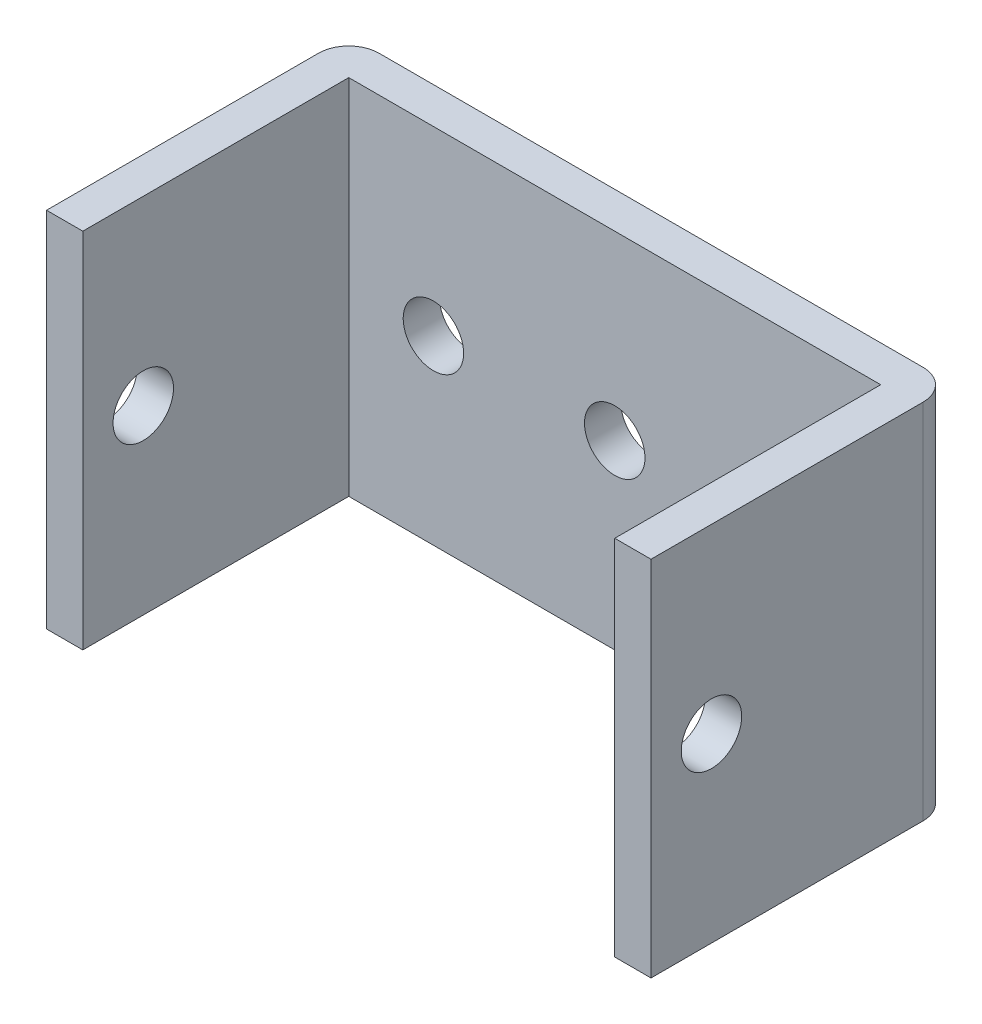
ISO-10303-21;
HEADER;
FILE_DESCRIPTION(('STEP AP214'),'2;1');
FILE_NAME('part.step','',(''),(''),'','','');
FILE_SCHEMA(('AUTOMOTIVE_DESIGN { 1 0 10303 214 1 1 1 1 }'));
ENDSEC;
DATA;
#1=APPLICATION_CONTEXT('core data for automotive mechanical design processes');
#2=APPLICATION_PROTOCOL_DEFINITION('international standard','automotive_design',2000,#1);
#3=PRODUCT_CONTEXT('',#1,'mechanical');
#4=PRODUCT('Part','Part','',(#3));
#5=PRODUCT_RELATED_PRODUCT_CATEGORY('part','',(#4));
#6=PRODUCT_DEFINITION_FORMATION('','',#4);
#7=PRODUCT_DEFINITION_CONTEXT('part definition',#1,'design');
#8=PRODUCT_DEFINITION('design','',#6,#7);
#9=PRODUCT_DEFINITION_SHAPE('','',#8);
#10=(LENGTH_UNIT() NAMED_UNIT(*) SI_UNIT(.MILLI.,.METRE.));
#11=(NAMED_UNIT(*) PLANE_ANGLE_UNIT() SI_UNIT($,.RADIAN.));
#12=(NAMED_UNIT(*) SI_UNIT($,.STERADIAN.) SOLID_ANGLE_UNIT());
#13=UNCERTAINTY_MEASURE_WITH_UNIT(LENGTH_MEASURE(1.E-05),#10,'distance_accuracy_value','');
#14=(GEOMETRIC_REPRESENTATION_CONTEXT(3) GLOBAL_UNCERTAINTY_ASSIGNED_CONTEXT((#13)) GLOBAL_UNIT_ASSIGNED_CONTEXT((#10,
#11,#12)) REPRESENTATION_CONTEXT('',''));
#15=CARTESIAN_POINT('',(0.,0.,0.));
#16=DIRECTION('',(0.,0.,1.));
#17=DIRECTION('',(1.,0.,0.));
#18=AXIS2_PLACEMENT_3D('',#15,#16,#17);
#19=CARTESIAN_POINT('',(6.,-30.,0.));
#20=DIRECTION('',(0.,0.,1.));
#21=DIRECTION('',(1.,0.,0.));
#22=AXIS2_PLACEMENT_3D('',#19,#20,#21);
#23=PLANE('',#22);
#24=DIRECTION('',(1.,0.,0.));
#25=VECTOR('',#24,1.);
#26=CARTESIAN_POINT('',(6.,30.,0.));
#27=LINE('',#26,#25);
#28=CARTESIAN_POINT('',(0.,30.,0.));
#29=VERTEX_POINT('',#28);
#30=CARTESIAN_POINT('',(6.,30.,0.));
#31=VERTEX_POINT('',#30);
#32=EDGE_CURVE('E161',#29,#31,#27,.T.);
#33=ORIENTED_EDGE('',*,*,#32,.F.);
#34=DIRECTION('',(0.,1.,0.));
#35=VECTOR('',#34,1.);
#36=CARTESIAN_POINT('',(0.,-30.,0.));
#37=LINE('',#36,#35);
#38=CARTESIAN_POINT('',(0.,-30.,0.));
#39=VERTEX_POINT('',#38);
#40=EDGE_CURVE('E138',#39,#29,#37,.T.);
#41=ORIENTED_EDGE('',*,*,#40,.F.);
#42=DIRECTION('',(1.,0.,0.));
#43=VECTOR('',#42,1.);
#44=CARTESIAN_POINT('',(6.,-30.,0.));
#45=LINE('',#44,#43);
#46=CARTESIAN_POINT('',(6.,-30.,0.));
#47=VERTEX_POINT('',#46);
#48=EDGE_CURVE('E132',#39,#47,#45,.T.);
#49=ORIENTED_EDGE('',*,*,#48,.T.);
#50=DIRECTION('',(0.,1.,0.));
#51=VECTOR('',#50,1.);
#52=CARTESIAN_POINT('',(6.,-30.,0.));
#53=LINE('',#52,#51);
#54=EDGE_CURVE('E116',#47,#31,#53,.T.);
#55=ORIENTED_EDGE('',*,*,#54,.T.);
#56=EDGE_LOOP('',(#33,#41,#49,#55));
#57=FACE_BOUND('',#56,.T.);
#58=ADVANCED_FACE('F39',(#57),#23,.T.);
#59=CARTESIAN_POINT('',(0.,-30.,0.));
#60=DIRECTION('',(-1.,0.,0.));
#61=DIRECTION('',(0.,0.,1.));
#62=AXIS2_PLACEMENT_3D('',#59,#60,#61);
#63=PLANE('',#62);
#64=CARTESIAN_POINT('',(0.,0.,-10.));
#65=DIRECTION('',(-1.,0.,0.));
#66=DIRECTION('',(0.,0.,1.));
#67=AXIS2_PLACEMENT_3D('',#64,#65,#66);
#68=CIRCLE('',#67,5.);
#69=CARTESIAN_POINT('',(0.,0.,-15.));
#70=VERTEX_POINT('',#69);
#71=EDGE_CURVE('E205',#70,#70,#68,.F.);
#72=ORIENTED_EDGE('',*,*,#71,.T.);
#73=EDGE_LOOP('',(#72));
#74=FACE_BOUND('',#73,.T.);
#75=DIRECTION('',(0.,0.,1.));
#76=VECTOR('',#75,1.);
#77=CARTESIAN_POINT('',(0.,30.,0.));
#78=LINE('',#77,#76);
#79=CARTESIAN_POINT('',(0.,30.,-45.));
#80=VERTEX_POINT('',#79);
#81=EDGE_CURVE('E139',#80,#29,#78,.T.);
#82=ORIENTED_EDGE('',*,*,#81,.F.);
#83=DIRECTION('',(0.,1.,0.));
#84=VECTOR('',#83,1.);
#85=CARTESIAN_POINT('',(0.,-30.,-45.));
#86=LINE('',#85,#84);
#87=CARTESIAN_POINT('',(0.,-30.,-45.));
#88=VERTEX_POINT('',#87);
#89=EDGE_CURVE('E11',#80,#88,#86,.F.);
#90=ORIENTED_EDGE('',*,*,#89,.T.);
#91=DIRECTION('',(0.,0.,1.));
#92=VECTOR('',#91,1.);
#93=CARTESIAN_POINT('',(0.,-30.,0.));
#94=LINE('',#93,#92);
#95=EDGE_CURVE('E130',#88,#39,#94,.T.);
#96=ORIENTED_EDGE('',*,*,#95,.T.);
#97=ORIENTED_EDGE('',*,*,#40,.T.);
#98=EDGE_LOOP('',(#82,#90,#96,#97));
#99=FACE_BOUND('',#98,.T.);
#100=ADVANCED_FACE('F231',(#74,#99),#63,.T.);
#101=CARTESIAN_POINT('',(0.,-30.,-50.));
#102=DIRECTION('',(0.,0.,-1.));
#103=DIRECTION('',(-1.,0.,0.));
#104=AXIS2_PLACEMENT_3D('',#101,#102,#103);
#105=PLANE('',#104);
#106=CARTESIAN_POINT('',(80.,0.,-50.));
#107=DIRECTION('',(0.,0.,-1.));
#108=DIRECTION('',(-1.,0.,0.));
#109=AXIS2_PLACEMENT_3D('',#106,#107,#108);
#110=CIRCLE('',#109,4.99999999999999);
#111=CARTESIAN_POINT('',(75.,0.,-50.));
#112=VERTEX_POINT('',#111);
#113=EDGE_CURVE('E144',#112,#112,#110,.T.);
#114=ORIENTED_EDGE('',*,*,#113,.F.);
#115=EDGE_LOOP('',(#114));
#116=FACE_BOUND('',#115,.T.);
#117=CARTESIAN_POINT('',(20.,0.,-50.));
#118=DIRECTION('',(0.,0.,-1.));
#119=DIRECTION('',(-1.,0.,0.));
#120=AXIS2_PLACEMENT_3D('',#117,#118,#119);
#121=CIRCLE('',#120,5.);
#122=CARTESIAN_POINT('',(15.,0.,-50.));
#123=VERTEX_POINT('',#122);
#124=EDGE_CURVE('E194',#123,#123,#121,.T.);
#125=ORIENTED_EDGE('',*,*,#124,.F.);
#126=EDGE_LOOP('',(#125));
#127=FACE_BOUND('',#126,.T.);
#128=CARTESIAN_POINT('',(50.,0.,-50.));
#129=DIRECTION('',(0.,0.,-1.));
#130=DIRECTION('',(-1.,0.,0.));
#131=AXIS2_PLACEMENT_3D('',#128,#129,#130);
#132=CIRCLE('',#131,5.00000000000002);
#133=CARTESIAN_POINT('',(45.,0.,-50.));
#134=VERTEX_POINT('',#133);
#135=EDGE_CURVE('E190',#134,#134,#132,.T.);
#136=ORIENTED_EDGE('',*,*,#135,.F.);
#137=EDGE_LOOP('',(#136));
#138=FACE_BOUND('',#137,.T.);
#139=DIRECTION('',(-1.,0.,0.));
#140=VECTOR('',#139,1.);
#141=CARTESIAN_POINT('',(0.,30.,-50.));
#142=LINE('',#141,#140);
#143=CARTESIAN_POINT('',(95.,30.,-50.));
#144=VERTEX_POINT('',#143);
#145=CARTESIAN_POINT('',(5.,30.,-50.));
#146=VERTEX_POINT('',#145);
#147=EDGE_CURVE('E142',#144,#146,#142,.T.);
#148=ORIENTED_EDGE('',*,*,#147,.F.);
#149=DIRECTION('',(0.,1.,0.));
#150=VECTOR('',#149,1.);
#151=CARTESIAN_POINT('',(95.,-30.,-50.));
#152=LINE('',#151,#150);
#153=CARTESIAN_POINT('',(95.,-30.,-50.));
#154=VERTEX_POINT('',#153);
#155=EDGE_CURVE('E215',#144,#154,#152,.F.);
#156=ORIENTED_EDGE('',*,*,#155,.T.);
#157=DIRECTION('',(-1.,0.,0.));
#158=VECTOR('',#157,1.);
#159=CARTESIAN_POINT('',(0.,-30.,-50.));
#160=LINE('',#159,#158);
#161=CARTESIAN_POINT('',(5.,-30.,-50.));
#162=VERTEX_POINT('',#161);
#163=EDGE_CURVE('E158',#154,#162,#160,.T.);
#164=ORIENTED_EDGE('',*,*,#163,.T.);
#165=DIRECTION('',(0.,1.,0.));
#166=VECTOR('',#165,1.);
#167=CARTESIAN_POINT('',(5.,-30.,-50.));
#168=LINE('',#167,#166);
#169=EDGE_CURVE('E207',#162,#146,#168,.T.);
#170=ORIENTED_EDGE('',*,*,#169,.T.);
#171=EDGE_LOOP('',(#148,#156,#164,#170));
#172=FACE_BOUND('',#171,.T.);
#173=ADVANCED_FACE('F229',(#116,#127,#138,#172),#105,.T.);
#174=CARTESIAN_POINT('',(100.,-30.,-50.));
#175=DIRECTION('',(1.,0.,0.));
#176=DIRECTION('',(0.,0.,-1.));
#177=AXIS2_PLACEMENT_3D('',#174,#175,#176);
#178=PLANE('',#177);
#179=CARTESIAN_POINT('',(100.,0.,-10.));
#180=DIRECTION('',(1.,0.,0.));
#181=DIRECTION('',(0.,0.,-1.));
#182=AXIS2_PLACEMENT_3D('',#179,#180,#181);
#183=CIRCLE('',#182,5.);
#184=CARTESIAN_POINT('',(100.,0.,-15.));
#185=VERTEX_POINT('',#184);
#186=EDGE_CURVE('E330',#185,#185,#183,.T.);
#187=ORIENTED_EDGE('',*,*,#186,.F.);
#188=EDGE_LOOP('',(#187));
#189=FACE_BOUND('',#188,.T.);
#190=DIRECTION('',(0.,0.,-1.));
#191=VECTOR('',#190,1.);
#192=CARTESIAN_POINT('',(100.,-30.,-50.));
#193=LINE('',#192,#191);
#194=CARTESIAN_POINT('',(100.,-30.,0.));
#195=VERTEX_POINT('',#194);
#196=CARTESIAN_POINT('',(100.,-30.,-45.));
#197=VERTEX_POINT('',#196);
#198=EDGE_CURVE('E154',#195,#197,#193,.T.);
#199=ORIENTED_EDGE('',*,*,#198,.T.);
#200=DIRECTION('',(0.,1.,0.));
#201=VECTOR('',#200,1.);
#202=CARTESIAN_POINT('',(100.,-30.,-45.));
#203=LINE('',#202,#201);
#204=CARTESIAN_POINT('',(100.,30.,-45.));
#205=VERTEX_POINT('',#204);
#206=EDGE_CURVE('E178',#197,#205,#203,.T.);
#207=ORIENTED_EDGE('',*,*,#206,.T.);
#208=DIRECTION('',(0.,0.,-1.));
#209=VECTOR('',#208,1.);
#210=CARTESIAN_POINT('',(100.,30.,-50.));
#211=LINE('',#210,#209);
#212=CARTESIAN_POINT('',(100.,30.,0.));
#213=VERTEX_POINT('',#212);
#214=EDGE_CURVE('E174',#213,#205,#211,.T.);
#215=ORIENTED_EDGE('',*,*,#214,.F.);
#216=DIRECTION('',(0.,1.,0.));
#217=VECTOR('',#216,1.);
#218=CARTESIAN_POINT('',(100.,-30.,0.));
#219=LINE('',#218,#217);
#220=EDGE_CURVE('E179',#195,#213,#219,.T.);
#221=ORIENTED_EDGE('',*,*,#220,.F.);
#222=EDGE_LOOP('',(#199,#207,#215,#221));
#223=FACE_BOUND('',#222,.T.);
#224=ADVANCED_FACE('F222',(#189,#223),#178,.T.);
#225=CARTESIAN_POINT('',(100.,-30.,0.));
#226=DIRECTION('',(0.,0.,1.));
#227=DIRECTION('',(1.,0.,0.));
#228=AXIS2_PLACEMENT_3D('',#225,#226,#227);
#229=PLANE('',#228);
#230=DIRECTION('',(1.,0.,0.));
#231=VECTOR('',#230,1.);
#232=CARTESIAN_POINT('',(100.,30.,0.));
#233=LINE('',#232,#231);
#234=CARTESIAN_POINT('',(94.,30.,0.));
#235=VERTEX_POINT('',#234);
#236=EDGE_CURVE('E168',#235,#213,#233,.T.);
#237=ORIENTED_EDGE('',*,*,#236,.F.);
#238=DIRECTION('',(0.,1.,0.));
#239=VECTOR('',#238,1.);
#240=CARTESIAN_POINT('',(94.,-30.,0.));
#241=LINE('',#240,#239);
#242=CARTESIAN_POINT('',(94.,-30.,0.));
#243=VERTEX_POINT('',#242);
#244=EDGE_CURVE('E185',#243,#235,#241,.T.);
#245=ORIENTED_EDGE('',*,*,#244,.F.);
#246=DIRECTION('',(1.,0.,0.));
#247=VECTOR('',#246,1.);
#248=CARTESIAN_POINT('',(100.,-30.,0.));
#249=LINE('',#248,#247);
#250=EDGE_CURVE('E155',#243,#195,#249,.T.);
#251=ORIENTED_EDGE('',*,*,#250,.T.);
#252=ORIENTED_EDGE('',*,*,#220,.T.);
#253=EDGE_LOOP('',(#237,#245,#251,#252));
#254=FACE_BOUND('',#253,.T.);
#255=ADVANCED_FACE('F238',(#254),#229,.T.);
#256=CARTESIAN_POINT('',(94.,-30.,0.));
#257=DIRECTION('',(-1.,0.,0.));
#258=DIRECTION('',(0.,0.,1.));
#259=AXIS2_PLACEMENT_3D('',#256,#257,#258);
#260=PLANE('',#259);
#261=CARTESIAN_POINT('',(94.,0.,-10.));
#262=DIRECTION('',(-1.,0.,0.));
#263=DIRECTION('',(0.,0.,1.));
#264=AXIS2_PLACEMENT_3D('',#261,#262,#263);
#265=CIRCLE('',#264,5.);
#266=CARTESIAN_POINT('',(94.,0.,-15.));
#267=VERTEX_POINT('',#266);
#268=EDGE_CURVE('E191',#267,#267,#265,.T.);
#269=ORIENTED_EDGE('',*,*,#268,.F.);
#270=EDGE_LOOP('',(#269));
#271=FACE_BOUND('',#270,.T.);
#272=DIRECTION('',(0.,0.,1.));
#273=VECTOR('',#272,1.);
#274=CARTESIAN_POINT('',(94.,30.,0.));
#275=LINE('',#274,#273);
#276=CARTESIAN_POINT('',(94.,30.,-44.));
#277=VERTEX_POINT('',#276);
#278=EDGE_CURVE('E170',#277,#235,#275,.T.);
#279=ORIENTED_EDGE('',*,*,#278,.F.);
#280=DIRECTION('',(0.,1.,0.));
#281=VECTOR('',#280,1.);
#282=CARTESIAN_POINT('',(94.,-30.,-44.));
#283=LINE('',#282,#281);
#284=CARTESIAN_POINT('',(94.,-30.,-44.));
#285=VERTEX_POINT('',#284);
#286=EDGE_CURVE('E184',#285,#277,#283,.T.);
#287=ORIENTED_EDGE('',*,*,#286,.F.);
#288=DIRECTION('',(0.,0.,1.));
#289=VECTOR('',#288,1.);
#290=CARTESIAN_POINT('',(94.,-30.,0.));
#291=LINE('',#290,#289);
#292=EDGE_CURVE('E149',#285,#243,#291,.T.);
#293=ORIENTED_EDGE('',*,*,#292,.T.);
#294=ORIENTED_EDGE('',*,*,#244,.T.);
#295=EDGE_LOOP('',(#279,#287,#293,#294));
#296=FACE_BOUND('',#295,.T.);
#297=ADVANCED_FACE('F240',(#271,#296),#260,.T.);
#298=CARTESIAN_POINT('',(94.,-30.,-44.));
#299=DIRECTION('',(0.,0.,1.));
#300=DIRECTION('',(1.,0.,0.));
#301=AXIS2_PLACEMENT_3D('',#298,#299,#300);
#302=PLANE('',#301);
#303=CARTESIAN_POINT('',(80.,0.,-44.));
#304=DIRECTION('',(0.,0.,1.));
#305=DIRECTION('',(1.,0.,0.));
#306=AXIS2_PLACEMENT_3D('',#303,#304,#305);
#307=CIRCLE('',#306,4.99999999999999);
#308=CARTESIAN_POINT('',(85.,0.,-44.));
#309=VERTEX_POINT('',#308);
#310=EDGE_CURVE('E198',#309,#309,#307,.T.);
#311=ORIENTED_EDGE('',*,*,#310,.F.);
#312=EDGE_LOOP('',(#311));
#313=FACE_BOUND('',#312,.T.);
#314=CARTESIAN_POINT('',(20.,0.,-44.));
#315=DIRECTION('',(0.,0.,1.));
#316=DIRECTION('',(1.,0.,0.));
#317=AXIS2_PLACEMENT_3D('',#314,#315,#316);
#318=CIRCLE('',#317,5.);
#319=CARTESIAN_POINT('',(25.,0.,-44.));
#320=VERTEX_POINT('',#319);
#321=EDGE_CURVE('E195',#320,#320,#318,.T.);
#322=ORIENTED_EDGE('',*,*,#321,.F.);
#323=EDGE_LOOP('',(#322));
#324=FACE_BOUND('',#323,.T.);
#325=CARTESIAN_POINT('',(50.,0.,-44.));
#326=DIRECTION('',(0.,0.,1.));
#327=DIRECTION('',(1.,0.,0.));
#328=AXIS2_PLACEMENT_3D('',#325,#326,#327);
#329=CIRCLE('',#328,5.00000000000002);
#330=CARTESIAN_POINT('',(55.,0.,-44.));
#331=VERTEX_POINT('',#330);
#332=EDGE_CURVE('E187',#331,#331,#329,.T.);
#333=ORIENTED_EDGE('',*,*,#332,.F.);
#334=EDGE_LOOP('',(#333));
#335=FACE_BOUND('',#334,.T.);
#336=DIRECTION('',(1.,0.,0.));
#337=VECTOR('',#336,1.);
#338=CARTESIAN_POINT('',(94.,30.,-44.));
#339=LINE('',#338,#337);
#340=CARTESIAN_POINT('',(6.00000000000001,30.,-44.));
#341=VERTEX_POINT('',#340);
#342=EDGE_CURVE('E163',#341,#277,#339,.T.);
#343=ORIENTED_EDGE('',*,*,#342,.F.);
#344=DIRECTION('',(0.,1.,0.));
#345=VECTOR('',#344,1.);
#346=CARTESIAN_POINT('',(6.00000000000001,-30.,-44.));
#347=LINE('',#346,#345);
#348=CARTESIAN_POINT('',(6.00000000000001,-30.,-44.));
#349=VERTEX_POINT('',#348);
#350=EDGE_CURVE('E127',#349,#341,#347,.T.);
#351=ORIENTED_EDGE('',*,*,#350,.F.);
#352=DIRECTION('',(1.,0.,0.));
#353=VECTOR('',#352,1.);
#354=CARTESIAN_POINT('',(94.,-30.,-44.));
#355=LINE('',#354,#353);
#356=EDGE_CURVE('E135',#349,#285,#355,.T.);
#357=ORIENTED_EDGE('',*,*,#356,.T.);
#358=ORIENTED_EDGE('',*,*,#286,.T.);
#359=EDGE_LOOP('',(#343,#351,#357,#358));
#360=FACE_BOUND('',#359,.T.);
#361=ADVANCED_FACE('F234',(#313,#324,#335,#360),#302,.T.);
#362=CARTESIAN_POINT('',(6.00000000000001,-30.,-44.));
#363=DIRECTION('',(1.,0.,0.));
#364=DIRECTION('',(0.,0.,-1.));
#365=AXIS2_PLACEMENT_3D('',#362,#363,#364);
#366=PLANE('',#365);
#367=CARTESIAN_POINT('',(6.00000000000001,0.,-10.));
#368=DIRECTION('',(1.,0.,0.));
#369=DIRECTION('',(0.,0.,-1.));
#370=AXIS2_PLACEMENT_3D('',#367,#368,#369);
#371=CIRCLE('',#370,5.);
#372=CARTESIAN_POINT('',(6.00000000000001,0.,-15.));
#373=VERTEX_POINT('',#372);
#374=EDGE_CURVE('E200',#373,#373,#371,.T.);
#375=ORIENTED_EDGE('',*,*,#374,.F.);
#376=EDGE_LOOP('',(#375));
#377=FACE_BOUND('',#376,.T.);
#378=DIRECTION('',(0.,0.,-1.));
#379=VECTOR('',#378,1.);
#380=CARTESIAN_POINT('',(6.00000000000001,30.,-44.));
#381=LINE('',#380,#379);
#382=EDGE_CURVE('E121',#31,#341,#381,.T.);
#383=ORIENTED_EDGE('',*,*,#382,.F.);
#384=ORIENTED_EDGE('',*,*,#54,.F.);
#385=DIRECTION('',(0.,0.,-1.));
#386=VECTOR('',#385,1.);
#387=CARTESIAN_POINT('',(6.00000000000001,-30.,-44.));
#388=LINE('',#387,#386);
#389=EDGE_CURVE('E118',#47,#349,#388,.T.);
#390=ORIENTED_EDGE('',*,*,#389,.T.);
#391=ORIENTED_EDGE('',*,*,#350,.T.);
#392=EDGE_LOOP('',(#383,#384,#390,#391));
#393=FACE_BOUND('',#392,.T.);
#394=ADVANCED_FACE('F119',(#377,#393),#366,.T.);
#395=CARTESIAN_POINT('',(0.,-30.,0.));
#396=DIRECTION('',(0.,-1.,0.));
#397=DIRECTION('',(0.,0.,-1.));
#398=AXIS2_PLACEMENT_3D('',#395,#396,#397);
#399=PLANE('',#398);
#400=ORIENTED_EDGE('',*,*,#163,.F.);
#401=CARTESIAN_POINT('',(95.,-30.,-45.));
#402=DIRECTION('',(0.,-1.,0.));
#403=DIRECTION('',(0.,0.,-1.));
#404=AXIS2_PLACEMENT_3D('',#401,#402,#403);
#405=CIRCLE('',#404,5.);
#406=EDGE_CURVE('E50',#154,#197,#405,.T.);
#407=ORIENTED_EDGE('',*,*,#406,.T.);
#408=ORIENTED_EDGE('',*,*,#198,.F.);
#409=ORIENTED_EDGE('',*,*,#250,.F.);
#410=ORIENTED_EDGE('',*,*,#292,.F.);
#411=ORIENTED_EDGE('',*,*,#356,.F.);
#412=ORIENTED_EDGE('',*,*,#389,.F.);
#413=ORIENTED_EDGE('',*,*,#48,.F.);
#414=ORIENTED_EDGE('',*,*,#95,.F.);
#415=CARTESIAN_POINT('',(5.,-30.,-45.));
#416=DIRECTION('',(0.,-1.,0.));
#417=DIRECTION('',(0.,0.,-1.));
#418=AXIS2_PLACEMENT_3D('',#415,#416,#417);
#419=CIRCLE('',#418,5.);
#420=EDGE_CURVE('E56',#88,#162,#419,.T.);
#421=ORIENTED_EDGE('',*,*,#420,.T.);
#422=EDGE_LOOP('',(#400,#407,#408,#409,#410,#411,#412,#413,#414,#421));
#423=FACE_BOUND('',#422,.T.);
#424=ADVANCED_FACE('F131',(#423),#399,.T.);
#425=CARTESIAN_POINT('',(0.,30.,0.));
#426=DIRECTION('',(0.,-1.,0.));
#427=DIRECTION('',(0.,0.,-1.));
#428=AXIS2_PLACEMENT_3D('',#425,#426,#427);
#429=PLANE('',#428);
#430=ORIENTED_EDGE('',*,*,#214,.T.);
#431=CARTESIAN_POINT('',(95.,30.,-45.));
#432=DIRECTION('',(0.,-1.,0.));
#433=DIRECTION('',(0.,0.,-1.));
#434=AXIS2_PLACEMENT_3D('',#431,#432,#433);
#435=CIRCLE('',#434,5.);
#436=EDGE_CURVE('E210',#205,#144,#435,.F.);
#437=ORIENTED_EDGE('',*,*,#436,.T.);
#438=ORIENTED_EDGE('',*,*,#147,.T.);
#439=CARTESIAN_POINT('',(5.,30.,-45.));
#440=DIRECTION('',(0.,-1.,0.));
#441=DIRECTION('',(0.,0.,-1.));
#442=AXIS2_PLACEMENT_3D('',#439,#440,#441);
#443=CIRCLE('',#442,5.);
#444=EDGE_CURVE('E202',#146,#80,#443,.F.);
#445=ORIENTED_EDGE('',*,*,#444,.T.);
#446=ORIENTED_EDGE('',*,*,#81,.T.);
#447=ORIENTED_EDGE('',*,*,#32,.T.);
#448=ORIENTED_EDGE('',*,*,#382,.T.);
#449=ORIENTED_EDGE('',*,*,#342,.T.);
#450=ORIENTED_EDGE('',*,*,#278,.T.);
#451=ORIENTED_EDGE('',*,*,#236,.T.);
#452=EDGE_LOOP('',(#430,#437,#438,#445,#446,#447,#448,#449,#450,#451));
#453=FACE_BOUND('',#452,.T.);
#454=ADVANCED_FACE('F226',(#453),#429,.F.);
#455=CARTESIAN_POINT('',(50.,0.,-20.));
#456=DIRECTION('',(0.,0.,-1.));
#457=DIRECTION('',(-1.,0.,0.));
#458=AXIS2_PLACEMENT_3D('',#455,#456,#457);
#459=CYLINDRICAL_SURFACE('',#458,5.00000000000002);
#460=ORIENTED_EDGE('',*,*,#135,.T.);
#461=EDGE_LOOP('',(#460));
#462=FACE_BOUND('',#461,.T.);
#463=ORIENTED_EDGE('',*,*,#332,.T.);
#464=EDGE_LOOP('',(#463));
#465=FACE_BOUND('',#464,.T.);
#466=ADVANCED_FACE('F282',(#462,#465),#459,.F.);
#467=CARTESIAN_POINT('',(20.,0.,-20.));
#468=DIRECTION('',(0.,0.,-1.));
#469=DIRECTION('',(-1.,0.,0.));
#470=AXIS2_PLACEMENT_3D('',#467,#468,#469);
#471=CYLINDRICAL_SURFACE('',#470,5.);
#472=ORIENTED_EDGE('',*,*,#124,.T.);
#473=EDGE_LOOP('',(#472));
#474=FACE_BOUND('',#473,.T.);
#475=ORIENTED_EDGE('',*,*,#321,.T.);
#476=EDGE_LOOP('',(#475));
#477=FACE_BOUND('',#476,.T.);
#478=ADVANCED_FACE('F276',(#474,#477),#471,.F.);
#479=CARTESIAN_POINT('',(80.,0.,-20.));
#480=DIRECTION('',(0.,0.,-1.));
#481=DIRECTION('',(-1.,0.,0.));
#482=AXIS2_PLACEMENT_3D('',#479,#480,#481);
#483=CYLINDRICAL_SURFACE('',#482,4.99999999999999);
#484=ORIENTED_EDGE('',*,*,#113,.T.);
#485=EDGE_LOOP('',(#484));
#486=FACE_BOUND('',#485,.T.);
#487=ORIENTED_EDGE('',*,*,#310,.T.);
#488=EDGE_LOOP('',(#487));
#489=FACE_BOUND('',#488,.T.);
#490=ADVANCED_FACE('F273',(#486,#489),#483,.F.);
#491=CARTESIAN_POINT('',(-14.142135623731,0.,-10.));
#492=DIRECTION('',(1.,0.,0.));
#493=DIRECTION('',(0.,0.,-1.));
#494=AXIS2_PLACEMENT_3D('',#491,#492,#493);
#495=CYLINDRICAL_SURFACE('',#494,5.);
#496=CARTESIAN_POINT('',(6.00000000000001,0.,-15.));
#497=CARTESIAN_POINT('',(5.93750000000001,0.,-15.));
#498=CARTESIAN_POINT('',(5.87500000000001,0.,-15.));
#499=CARTESIAN_POINT('',(5.75000000000001,0.,-15.));
#500=CARTESIAN_POINT('',(5.68750000000001,0.,-15.));
#501=CARTESIAN_POINT('',(5.56250000000001,0.,-15.));
#502=CARTESIAN_POINT('',(5.50000000000001,0.,-15.));
#503=CARTESIAN_POINT('',(5.37500000000001,0.,-15.));
#504=CARTESIAN_POINT('',(5.31250000000001,0.,-15.));
#505=CARTESIAN_POINT('',(5.18750000000001,0.,-15.));
#506=CARTESIAN_POINT('',(5.12500000000001,0.,-15.));
#507=CARTESIAN_POINT('',(5.00000000000001,0.,-15.));
#508=CARTESIAN_POINT('',(4.93750000000001,0.,-15.));
#509=CARTESIAN_POINT('',(4.81250000000001,0.,-15.));
#510=CARTESIAN_POINT('',(4.75000000000001,0.,-15.));
#511=CARTESIAN_POINT('',(4.62500000000001,0.,-15.));
#512=CARTESIAN_POINT('',(4.56250000000001,0.,-15.));
#513=CARTESIAN_POINT('',(4.43750000000001,0.,-15.));
#514=CARTESIAN_POINT('',(4.37500000000001,0.,-15.));
#515=CARTESIAN_POINT('',(4.25000000000001,0.,-15.));
#516=CARTESIAN_POINT('',(4.18750000000001,0.,-15.));
#517=CARTESIAN_POINT('',(4.06250000000001,0.,-15.));
#518=CARTESIAN_POINT('',(4.00000000000001,0.,-15.));
#519=CARTESIAN_POINT('',(3.87500000000001,0.,-15.));
#520=CARTESIAN_POINT('',(3.81250000000001,0.,-15.));
#521=CARTESIAN_POINT('',(3.68750000000001,0.,-15.));
#522=CARTESIAN_POINT('',(3.62500000000001,0.,-15.));
#523=CARTESIAN_POINT('',(3.50000000000001,0.,-15.));
#524=CARTESIAN_POINT('',(3.43750000000001,0.,-15.));
#525=CARTESIAN_POINT('',(3.31250000000001,0.,-15.));
#526=CARTESIAN_POINT('',(3.25000000000001,0.,-15.));
#527=CARTESIAN_POINT('',(3.12500000000001,0.,-15.));
#528=CARTESIAN_POINT('',(3.06250000000001,0.,-15.));
#529=CARTESIAN_POINT('',(2.93750000000001,0.,-15.));
#530=CARTESIAN_POINT('',(2.87500000000001,0.,-15.));
#531=CARTESIAN_POINT('',(2.75000000000001,0.,-15.));
#532=CARTESIAN_POINT('',(2.68750000000001,0.,-15.));
#533=CARTESIAN_POINT('',(2.5625,0.,-15.));
#534=CARTESIAN_POINT('',(2.5,0.,-15.));
#535=CARTESIAN_POINT('',(2.375,0.,-15.));
#536=CARTESIAN_POINT('',(2.3125,0.,-15.));
#537=CARTESIAN_POINT('',(2.1875,0.,-15.));
#538=CARTESIAN_POINT('',(2.125,0.,-15.));
#539=CARTESIAN_POINT('',(2.,0.,-15.));
#540=CARTESIAN_POINT('',(1.9375,0.,-15.));
#541=CARTESIAN_POINT('',(1.8125,0.,-15.));
#542=CARTESIAN_POINT('',(1.75,0.,-15.));
#543=CARTESIAN_POINT('',(1.625,0.,-15.));
#544=CARTESIAN_POINT('',(1.5625,0.,-15.));
#545=CARTESIAN_POINT('',(1.4375,0.,-15.));
#546=CARTESIAN_POINT('',(1.375,0.,-15.));
#547=CARTESIAN_POINT('',(1.25,0.,-15.));
#548=CARTESIAN_POINT('',(1.1875,0.,-15.));
#549=CARTESIAN_POINT('',(1.0625,0.,-15.));
#550=CARTESIAN_POINT('',(1.,0.,-15.));
#551=CARTESIAN_POINT('',(0.875000000000003,0.,-15.));
#552=CARTESIAN_POINT('',(0.812500000000002,0.,-15.));
#553=CARTESIAN_POINT('',(0.687500000000002,0.,-15.));
#554=CARTESIAN_POINT('',(0.625000000000002,0.,-15.));
#555=CARTESIAN_POINT('',(0.500000000000002,0.,-15.));
#556=CARTESIAN_POINT('',(0.437500000000002,0.,-15.));
#557=CARTESIAN_POINT('',(0.312500000000002,0.,-15.));
#558=CARTESIAN_POINT('',(0.250000000000002,0.,-15.));
#559=CARTESIAN_POINT('',(0.125000000000002,0.,-15.));
#560=CARTESIAN_POINT('',(0.0625000000000018,0.,-15.));
#561=CARTESIAN_POINT('',(0.,0.,-15.));
#562=B_SPLINE_CURVE_WITH_KNOTS('',3,(#496,#497,#498,#499,#500,#501,#502,#503,#504,#505,#506,
#507,#508,#509,#510,#511,#512,#513,#514,#515,#516,#517,#518,#519,#520,#521,#522,#523,#524,#525,
#526,#527,#528,#529,#530,#531,#532,#533,#534,#535,#536,#537,#538,#539,#540,#541,#542,#543,#544,
#545,#546,#547,#548,#549,#550,#551,#552,#553,#554,#555,#556,#557,#558,#559,#560,#561),
.UNSPECIFIED.,.F.,.F.,(4,2,2,2,2,2,2,2,2,2,2,2,2,2,2,2,2,2,2,2,2,2,2,2,2,2,2,2,2,2,2,2,4),(0.,
0.1875,0.375,0.5625,0.750000000000001,0.937500000000001,1.125,1.3125,1.5,1.6875,1.875,2.0625,
2.25,2.4375,2.625,2.8125,3.,3.1875,3.375,3.56250000000001,3.75000000000001,3.93750000000001,
4.12500000000001,4.31250000000001,4.50000000000001,4.68750000000001,4.87500000000001,
5.06250000000001,5.25000000000001,5.43750000000001,5.62500000000001,5.81250000000001,
6.00000000000001),.UNSPECIFIED.);
#563=EDGE_CURVE('BSEAM268',#373,#70,#562,.T.);
#564=ORIENTED_EDGE('',*,*,#374,.T.);
#565=ORIENTED_EDGE('',*,*,#71,.F.);
#566=ORIENTED_EDGE('',*,*,#563,.T.);
#567=ORIENTED_EDGE('',*,*,#563,.F.);
#568=EDGE_LOOP('',(#564,#566,#565,#567));
#569=FACE_BOUND('',#568,.T.);
#570=ADVANCED_FACE('F268',(#569),#495,.F.);
#571=CARTESIAN_POINT('',(94.,0.,-15.));
#572=CARTESIAN_POINT('',(94.0625,0.,-15.));
#573=CARTESIAN_POINT('',(94.125,0.,-15.));
#574=CARTESIAN_POINT('',(94.25,0.,-15.));
#575=CARTESIAN_POINT('',(94.3125,0.,-15.));
#576=CARTESIAN_POINT('',(94.4375,0.,-15.));
#577=CARTESIAN_POINT('',(94.5,0.,-15.));
#578=CARTESIAN_POINT('',(94.625,0.,-15.));
#579=CARTESIAN_POINT('',(94.6875,0.,-15.));
#580=CARTESIAN_POINT('',(94.8125,0.,-15.));
#581=CARTESIAN_POINT('',(94.875,0.,-15.));
#582=CARTESIAN_POINT('',(95.,0.,-15.));
#583=CARTESIAN_POINT('',(95.0625,0.,-15.));
#584=CARTESIAN_POINT('',(95.1875,0.,-15.));
#585=CARTESIAN_POINT('',(95.25,0.,-15.));
#586=CARTESIAN_POINT('',(95.375,0.,-15.));
#587=CARTESIAN_POINT('',(95.4375,0.,-15.));
#588=CARTESIAN_POINT('',(95.5625,0.,-15.));
#589=CARTESIAN_POINT('',(95.625,0.,-15.));
#590=CARTESIAN_POINT('',(95.75,0.,-15.));
#591=CARTESIAN_POINT('',(95.8125,0.,-15.));
#592=CARTESIAN_POINT('',(95.9375,0.,-15.));
#593=CARTESIAN_POINT('',(96.,0.,-15.));
#594=CARTESIAN_POINT('',(96.125,0.,-15.));
#595=CARTESIAN_POINT('',(96.1875,0.,-15.));
#596=CARTESIAN_POINT('',(96.3125,0.,-15.));
#597=CARTESIAN_POINT('',(96.375,0.,-15.));
#598=CARTESIAN_POINT('',(96.5,0.,-15.));
#599=CARTESIAN_POINT('',(96.5625,0.,-15.));
#600=CARTESIAN_POINT('',(96.6875,0.,-15.));
#601=CARTESIAN_POINT('',(96.75,0.,-15.));
#602=CARTESIAN_POINT('',(96.875,0.,-15.));
#603=CARTESIAN_POINT('',(96.9375,0.,-15.));
#604=CARTESIAN_POINT('',(97.0625,0.,-15.));
#605=CARTESIAN_POINT('',(97.125,0.,-15.));
#606=CARTESIAN_POINT('',(97.25,0.,-15.));
#607=CARTESIAN_POINT('',(97.3125,0.,-15.));
#608=CARTESIAN_POINT('',(97.4375,0.,-15.));
#609=CARTESIAN_POINT('',(97.5,0.,-15.));
#610=CARTESIAN_POINT('',(97.625,0.,-15.));
#611=CARTESIAN_POINT('',(97.6875,0.,-15.));
#612=CARTESIAN_POINT('',(97.8125,0.,-15.));
#613=CARTESIAN_POINT('',(97.875,0.,-15.));
#614=CARTESIAN_POINT('',(98.,0.,-15.));
#615=CARTESIAN_POINT('',(98.0625,0.,-15.));
#616=CARTESIAN_POINT('',(98.1875,0.,-15.));
#617=CARTESIAN_POINT('',(98.25,0.,-15.));
#618=CARTESIAN_POINT('',(98.375,0.,-15.));
#619=CARTESIAN_POINT('',(98.4375,0.,-15.));
#620=CARTESIAN_POINT('',(98.5625,0.,-15.));
#621=CARTESIAN_POINT('',(98.625,0.,-15.));
#622=CARTESIAN_POINT('',(98.75,0.,-15.));
#623=CARTESIAN_POINT('',(98.8125,0.,-15.));
#624=CARTESIAN_POINT('',(98.9375,0.,-15.));
#625=CARTESIAN_POINT('',(99.,0.,-15.));
#626=CARTESIAN_POINT('',(99.125,0.,-15.));
#627=CARTESIAN_POINT('',(99.1875,0.,-15.));
#628=CARTESIAN_POINT('',(99.3125,0.,-15.));
#629=CARTESIAN_POINT('',(99.375,0.,-15.));
#630=CARTESIAN_POINT('',(99.5,0.,-15.));
#631=CARTESIAN_POINT('',(99.5625,0.,-15.));
#632=CARTESIAN_POINT('',(99.6875,0.,-15.));
#633=CARTESIAN_POINT('',(99.75,0.,-15.));
#634=CARTESIAN_POINT('',(99.875,0.,-15.));
#635=CARTESIAN_POINT('',(99.9375,0.,-15.));
#636=CARTESIAN_POINT('',(100.,0.,-15.));
#637=B_SPLINE_CURVE_WITH_KNOTS('',3,(#571,#572,#573,#574,#575,#576,#577,#578,#579,#580,#581,
#582,#583,#584,#585,#586,#587,#588,#589,#590,#591,#592,#593,#594,#595,#596,#597,#598,#599,#600,
#601,#602,#603,#604,#605,#606,#607,#608,#609,#610,#611,#612,#613,#614,#615,#616,#617,#618,#619,
#620,#621,#622,#623,#624,#625,#626,#627,#628,#629,#630,#631,#632,#633,#634,#635,#636),
.UNSPECIFIED.,.F.,.F.,(4,2,2,2,2,2,2,2,2,2,2,2,2,2,2,2,2,2,2,2,2,2,2,2,2,2,2,2,2,2,2,2,4),(0.,
0.187499999999993,0.375,0.562499999999994,0.750000000000001,0.937499999999994,1.125,
1.31249999999999,1.5,1.68749999999999,1.87499999999999,2.06249999999999,2.24999999999999,2.4375,
2.62499999999999,2.8125,2.99999999999999,3.18749999999998,3.37499999999999,3.56249999999998,
3.74999999999999,3.93749999999998,4.12499999999999,4.31249999999998,4.49999999999998,
4.68749999999998,4.87499999999998,5.06249999999998,5.24999999999998,5.43749999999998,
5.62499999999998,5.81249999999998,5.99999999999998),.UNSPECIFIED.);
#638=EDGE_CURVE('BSEAM265',#267,#185,#637,.T.);
#639=ORIENTED_EDGE('',*,*,#268,.T.);
#640=ORIENTED_EDGE('',*,*,#186,.T.);
#641=ORIENTED_EDGE('',*,*,#638,.T.);
#642=ORIENTED_EDGE('',*,*,#638,.F.);
#643=EDGE_LOOP('',(#639,#641,#640,#642));
#644=FACE_BOUND('',#643,.T.);
#645=ADVANCED_FACE('F265',(#644),#495,.F.);
#646=CARTESIAN_POINT('',(95.,-30.,-45.));
#647=DIRECTION('',(0.,1.,0.));
#648=DIRECTION('',(0.,0.,1.));
#649=AXIS2_PLACEMENT_3D('',#646,#647,#648);
#650=CYLINDRICAL_SURFACE('',#649,5.);
#651=ORIENTED_EDGE('',*,*,#406,.F.);
#652=ORIENTED_EDGE('',*,*,#155,.F.);
#653=ORIENTED_EDGE('',*,*,#436,.F.);
#654=ORIENTED_EDGE('',*,*,#206,.F.);
#655=EDGE_LOOP('',(#651,#652,#653,#654));
#656=FACE_BOUND('',#655,.T.);
#657=ADVANCED_FACE('F224',(#656),#650,.T.);
#658=CARTESIAN_POINT('',(5.,-30.,-45.));
#659=DIRECTION('',(0.,1.,0.));
#660=DIRECTION('',(0.,0.,1.));
#661=AXIS2_PLACEMENT_3D('',#658,#659,#660);
#662=CYLINDRICAL_SURFACE('',#661,5.);
#663=ORIENTED_EDGE('',*,*,#420,.F.);
#664=ORIENTED_EDGE('',*,*,#89,.F.);
#665=ORIENTED_EDGE('',*,*,#444,.F.);
#666=ORIENTED_EDGE('',*,*,#169,.F.);
#667=EDGE_LOOP('',(#663,#664,#665,#666));
#668=FACE_BOUND('',#667,.T.);
#669=ADVANCED_FACE('F41',(#668),#662,.T.);
#670=CLOSED_SHELL('',(#58,#100,#173,#224,#255,#297,#361,#394,#424,#454,#466,#478,#490,#570,#645,
#657,#669));
#671=MANIFOLD_SOLID_BREP('B2',#670);
#672=ADVANCED_BREP_SHAPE_REPRESENTATION('',(#18,#671),#14);
#673=SHAPE_DEFINITION_REPRESENTATION(#9,#672);
ENDSEC;
END-ISO-10303-21;
